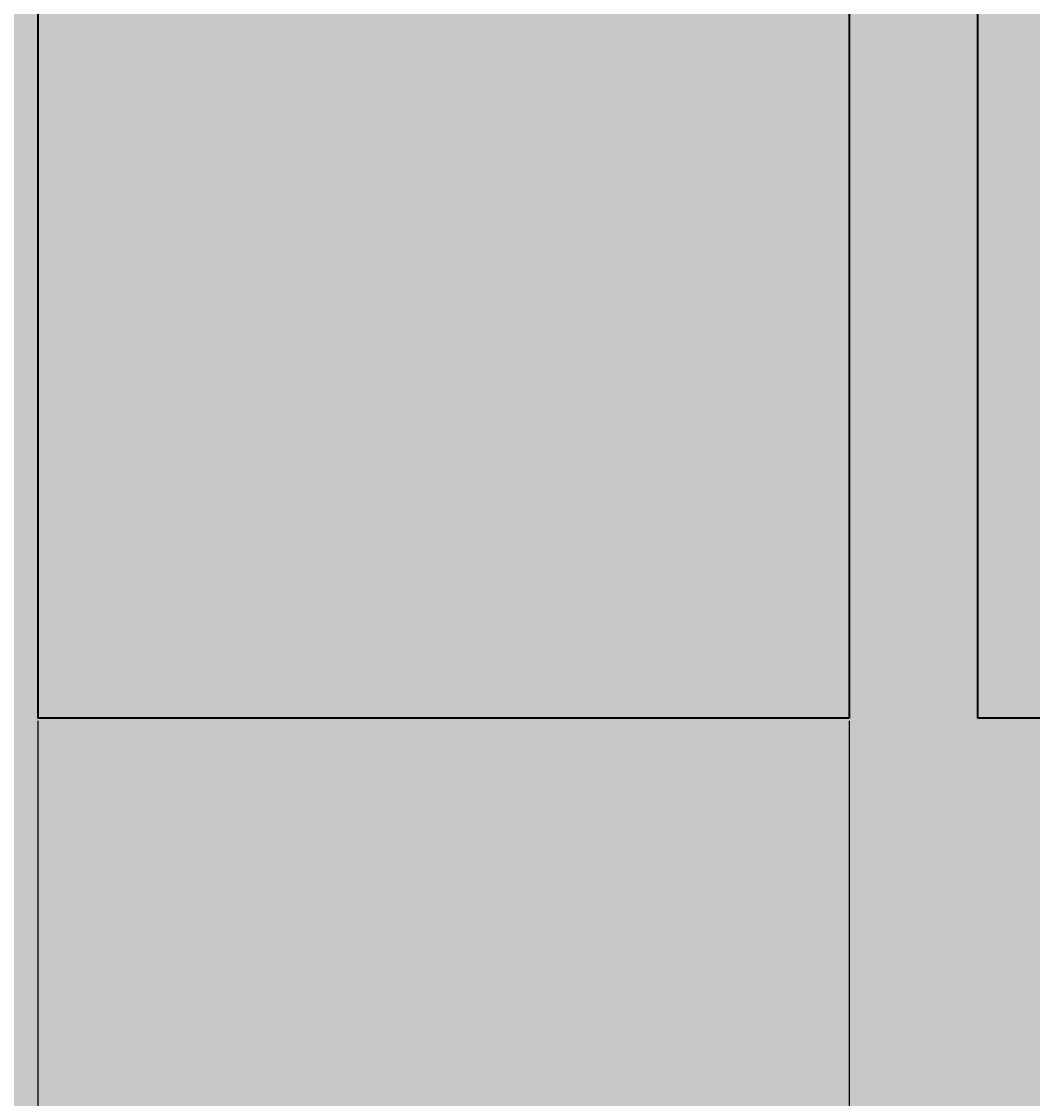
# Model space of a CAD drawing. Units: inches. Extents: x -1 to 292, y -3 to 199.
# Tile 20 of 52: x 82 to 106, y 42 to 68. Entities that reach past the tile are written whole.
import ezdxf

# ---------------------------------------------------------------- set-up
doc = ezdxf.new("R2010")
doc.units = ezdxf.units.IN
doc.header["$MEASUREMENT"] = 0
for name, color, linetype, lineweight in [('M-DIMS', 2, 'Continuous', 18), ('M-EQPM', 7, 'Continuous', 35), ('M-PATT', 8, 'Continuous', 13)]:
    doc.layers.add(name, color=color, linetype=linetype, lineweight=lineweight)
doc.styles.get("Standard").update_dxf_attribs({"font": 'arial.ttf'})
doc.dimstyles.get("Standard").update_dxf_attribs({"dimtxt": 0.18, "dimasz": 0.18, "dimexe": 0.18, "dimexo": 0.0625, "dimgap": 0.09, "dimtad": 0, "dimtih": 1, "dimtoh": 1, "dimdec": 4, "dimzin": 0, "dimdsep": 46, "dimtxsty": 'Standard', "dimcen": 0.09, "dimadec": 0, "dimazin": 0, "dimtfac": 1, "dimtdec": 4, "dimtofl": 0, "dimtmove": 0, "dimatfit": 3, "dimfxl": 1, "dimtolj": 1, "dimtzin": 0, "dimarcsym": 0})

# ---------------------------------------------------------------- blocks, each defined once
blk = doc.blocks.new('BOILER-TUBE')
blk.add_line((0, 40.63), (0, 0))
blk.add_lwpolyline([(3, 0), (0, 0)])
blk = doc.blocks.new('*D7')
at = {"layer": 'Defpoints', "color": 0, "transparency": 16777216}
for p in [(21.861, 54.582), (205.115, 54.582), (21.861, 39.982)]:
    blk.add_point(p, dxfattribs=at)
at = {"layer": 'M-DIMS', "color": 0, "lineweight": -2, "transparency": 16777216}
for p, q in [((21.861, 54.52), (21.861, 39.802)), ((205.115, 54.52), (205.115, 39.802)), ((22.041, 39.982), (113.033, 39.982)), ((204.935, 39.982), (113.944, 39.982))]:
    blk.add_line(p, q, dxfattribs=at)
at = {"layer": 'M-DIMS', "color": 0, "transparency": 16777216}
for points in [[(22.041, 40.012), (22.041, 39.952), (21.861, 39.982)], [(204.935, 40.012), (204.935, 39.952), (205.115, 39.982)]]:
    blk.add_solid(points, dxfattribs=at)
at = {"layer": 'M-DIMS', "color": 0, "transparency": 16777216, "insert": (113.488, 39.982), "char_height": 0.18, "attachment_point": 5}
blk.add_mtext('\\A1;183.25', dxfattribs=at)
blk = doc.blocks.new('*D8')
at = {"layer": 'Defpoints', "color": 0, "transparency": 16777216}
for p in [(-0.662, 126.765), (111.488, 126.765), (69.013, 25.514)]:
    blk.add_point(p, dxfattribs=at)
at = {"layer": 'M-DIMS', "color": 0, "lineweight": -2, "transparency": 16777216}
for p, q in [((111.426, 126.765), (-0.842, 126.765)), ((-0.662, 126.585), (-0.662, 76.321)), ((-0.662, 25.694), (-0.662, 75.958)), ((68.951, 25.514), (-0.842, 25.514))]:
    blk.add_line(p, q, dxfattribs=at)
at = {"layer": 'M-DIMS', "color": 0, "transparency": 16777216}
for points in [[(-0.692, 126.585), (-0.632, 126.585), (-0.662, 126.765)], [(-0.692, 25.694), (-0.632, 25.694), (-0.662, 25.514)]]:
    blk.add_solid(points, dxfattribs=at)
at = {"layer": 'M-DIMS', "color": 0, "transparency": 16777216, "insert": (-0.662, 76.14), "char_height": 0.18, "attachment_point": 5}
blk.add_mtext('\\A1;101.25', dxfattribs=at)
blk = doc.blocks.new('*D21')
at = {"layer": 'Defpoints', "color": 0, "transparency": 16777216}
for p in [(82.679, 51.267), (101.679, 51.267), (101.679, -2.71)]:
    blk.add_point(p, dxfattribs=at)
at = {"layer": 'M-DIMS', "color": 0, "lineweight": -2, "transparency": 16777216}
for p, q in [((82.679, 51.205), (82.679, -2.89)), ((101.679, 51.205), (101.679, -2.89)), ((82.859, -2.71), (91.968, -2.71)), ((101.499, -2.71), (92.389, -2.71))]:
    blk.add_line(p, q, dxfattribs=at)
at = {"layer": 'M-DIMS', "color": 0, "transparency": 16777216}
for points in [[(82.859, -2.68), (82.859, -2.74), (82.679, -2.71)], [(101.499, -2.68), (101.499, -2.74), (101.679, -2.71)]]:
    blk.add_solid(points, dxfattribs=at)
at = {"layer": 'M-DIMS', "color": 0, "transparency": 16777216, "insert": (92.179, -2.71), "char_height": 0.18, "attachment_point": 5}
blk.add_mtext('\\A1;19', dxfattribs=at)
blk = doc.blocks.new('*D22')
at = {"layer": 'Defpoints', "color": 0, "transparency": 16777216}
for p in [(82.679, 51.267), (122.679, 51.267), (122.679, -2.71)]:
    blk.add_point(p, dxfattribs=at)
at = {"layer": 'M-DIMS', "color": 0, "lineweight": -2, "transparency": 16777216}
for p, q in [((82.679, 51.205), (82.679, -2.89)), ((122.679, 51.205), (122.679, -2.89)), ((82.859, -2.71), (102.457, -2.71)), ((122.499, -2.71), (102.901, -2.71))]:
    blk.add_line(p, q, dxfattribs=at)
at = {"layer": 'M-DIMS', "color": 0, "transparency": 16777216}
for points in [[(82.859, -2.68), (82.859, -2.74), (82.679, -2.71)], [(122.499, -2.68), (122.499, -2.74), (122.679, -2.71)]]:
    blk.add_solid(points, dxfattribs=at)
at = {"layer": 'M-DIMS', "color": 0, "transparency": 16777216, "insert": (102.679, -2.71), "char_height": 0.18, "attachment_point": 5}
blk.add_mtext('\\A1;40', dxfattribs=at)

msp = doc.modelspace()

# ---------------------------------------------------------------- hatches: boundary and pattern name
at = {"layer": 'M-PATT'}
h = msp.add_hatch(color=256, dxfattribs=at)
h.set_gradient(color1=(237, 31, 36), color2=(242, 113, 114), tint=1, name='CYLINDER')
h.paths.add_polyline_path([(106.0735, 105.9941), (106.0735, 106.9941), (108.0603, 106.9941), (107.8488, 107.6501), (57.8007, 107.6501, 0.4142136), (49.9241, 99.7735), (52.3176, 101.3278), (55.0097, 99.7735), (57.4032, 101.3278), (60.0953, 99.7735), (62.4888, 101.3278), (65.1809, 99.7735), (67.5744, 101.3278), (70.2665, 99.7735), (72.66, 101.3278), (75.3521, 99.7735), (77.7456, 101.3278), (80.4377, 99.7735), (82.8312, 101.3278), (85.5233, 99.7735), (87.9168, 101.3278), (90.6089, 99.7735), (93.0024, 101.3278), (95.6945, 99.7735), (98.088, 101.3278), (100.7801, 99.7735), (103.1736, 101.3278), (105.8657, 99.7735), (108.2592, 101.3278), (110.9513, 99.7735), (113.3448, 101.3278), (116.0369, 99.7735), (118.4304, 101.3278), (121.1225, 99.7735), (123.516, 101.3278), (126.2082, 99.7735), (128.6016, 101.3278), (131.2938, 99.7735), (133.6872, 101.3278), (136.3794, 99.7735), (138.7728, 101.3278), (141.465, 99.7735), (143.8584, 101.3278), (146.5506, 99.7735), (148.944, 101.3278), (151.6362, 99.7735), (154.0296, 101.3278), (156.7218, 99.7735), (159.1152, 101.3278), (160.6222, 100.4578), (160.6222, 107.6501), (115.4883, 107.6501), (115.4883, 106.9941), (120.9032, 106.9941), (120.9032, 105.9941), (120.9032, 103.3981), (106.0735, 103.3981)])
h.paths.add_polyline_path([(169.176, 107.6501), (162.1623, 107.6501), (162.1623, 100.004), (164.2008, 101.3278), (166.893, 99.7735), (169.2864, 101.3278), (171.9786, 99.7735), (174.372, 101.3278), (177.0526, 99.7802, 0.4139642)])
h.paths.add_polyline_path([(111.4883, 107.6501), (107.8488, 107.6501), (108.0603, 106.9941), (111.4883, 106.9941)], flags=17)
h.paths.add_polyline_path([(61.6788, 91.897), (57.8007, 91.897, -0.1099266), (54.4604, 92.6403), (43.2011, 92.6403), (23.9502, 84.4688), (23.9502, 58.376), (43.2011, 47.2615), (50.9409, 47.2615, -0.2705926), (57.8007, 51.2672), (61.6788, 51.2672)])
h.paths.add_polyline_path([(73.6788, 91.897), (70.6788, 91.897), (70.6788, 51.2672), (73.6788, 51.2672)])
h.paths.add_polyline_path([(79.6788, 91.897), (76.6788, 91.897), (76.6788, 51.2672), (79.6788, 51.2672)])
h.paths.add_polyline_path([(67.6788, 91.897), (64.6788, 91.897), (64.6788, 51.2672), (67.6788, 51.2672)])
h.paths.add_polyline_path([(101.6788, 91.897), (82.6788, 91.897), (82.6788, 51.2672), (101.6788, 51.2672)])
h.paths.add_polyline_path([(107.6788, 91.897), (104.6788, 91.897), (104.6788, 51.2672), (107.6788, 51.2672)])
h.paths.add_polyline_path([(113.6788, 91.897), (110.6788, 91.897), (110.6788, 51.2672), (113.6788, 51.2672)])
h.paths.add_polyline_path([(119.6788, 91.897), (116.6788, 91.897), (116.6788, 51.2672), (119.6788, 51.2672)])
h.paths.add_polyline_path([(141.6788, 91.897), (122.6788, 91.897), (122.6788, 51.2672), (141.6788, 51.2672)])
h.paths.add_polyline_path([(147.6788, 91.897), (144.6788, 91.897), (144.6788, 51.2672), (147.6788, 51.2672)])
h.paths.add_polyline_path([(153.6788, 91.897), (150.6788, 91.897), (150.6788, 51.2672), (153.6788, 51.2672)])
h.paths.add_polyline_path([(159.6788, 91.897), (156.6788, 91.897), (156.6788, 51.2672), (159.6788, 51.2672)])
h.paths.add_polyline_path([(179.5897, 92.6403), (172.5163, 92.6403, -0.1099266), (169.176, 91.897), (162.6788, 91.897), (162.6788, 51.2672), (169.176, 51.2672, -0.2705926), (176.0358, 47.2615), (179.5897, 47.2615)])
h.paths.add_polyline_path([(203.0265, 84.4688), (183.7755, 92.6403), (181.5897, 92.6403), (181.5897, 47.2615), (183.7755, 47.2615), (203.0265, 58.376)])
h.paths.add_polyline_path([(184.4188, 61.52), (200.7224, 61.52), (200.7224, 77.7532), (184.4188, 77.7532)], flags=24)
h = msp.add_hatch(color=256, dxfattribs=at)
h.set_gradient(color1=(0, 255, 255), color2=(0, 255, 255), tint=1)
h.paths.add_polyline_path([(75.3521, 99.7735), (72.66, 101.3278), (70.2665, 99.7735), (67.5744, 101.3278), (65.1809, 99.7735), (62.4888, 101.3278), (60.0953, 99.7735), (57.4032, 101.3278), (55.0097, 99.7735), (52.3176, 101.3278), (49.9241, 99.7735, 0.4142136), (57.8007, 91.897), (61.6788, 91.897), (61.6788, 51.2672), (57.8007, 51.2672, 0.8088808), (54.5813, 36.2021), (65.0947, 51.2672), (64.6788, 51.2672), (64.6788, 91.897), (67.6788, 91.897), (67.6788, 51.2672), (65.0947, 51.2672), (54.5813, 36.2021, 0.1056561), (57.8007, 35.5141), (169.176, 35.5141, 1), (169.176, 51.2672), (162.6788, 51.2672), (162.6788, 91.897), (169.176, 91.897, 0.4144629), (177.0526, 99.7802), (174.372, 101.3278), (171.9786, 99.7735), (169.2864, 101.3278), (166.893, 99.7735), (164.2008, 101.3278), (162.1623, 100.004), (162.1623, 96.1027), (160.6222, 96.1027), (160.6222, 100.4578), (159.1152, 101.3278), (156.7218, 99.7735), (154.0296, 101.3278), (151.6362, 99.7735), (148.944, 101.3278), (146.5506, 99.7735), (143.8584, 101.3278), (141.465, 99.7735), (138.7728, 101.3278), (136.3794, 99.7735), (133.6872, 101.3278), (131.2938, 99.7735), (128.6016, 101.3278), (126.2082, 99.7735), (123.516, 101.3278), (121.1225, 99.7735), (118.4304, 101.3278), (116.0369, 99.7735), (113.3448, 101.3278), (110.9513, 99.7735), (108.2592, 101.3278), (105.8657, 99.7735), (103.1736, 101.3278), (100.7801, 99.7735), (98.088, 101.3278), (95.6945, 99.7735), (93.0024, 101.3278), (90.6089, 99.7735), (87.9168, 101.3278), (85.5233, 99.7735), (82.8312, 101.3278), (80.4377, 99.7735), (77.7456, 101.3278)])
h.paths.add_polyline_path([(79.6788, 91.897), (79.6788, 51.2672), (76.6788, 51.2672), (76.6788, 91.897)], flags=16)
h.paths.add_polyline_path([(73.6788, 91.897), (73.6788, 51.2672), (70.6788, 51.2672), (70.6788, 91.897)], flags=16)
h.paths.add_polyline_path([(82.6788, 91.897), (101.6788, 91.897), (101.6788, 51.2672), (82.6788, 51.2672)], flags=16)
h.paths.add_polyline_path([(104.6788, 91.897), (107.6788, 91.897), (107.6788, 51.2672), (104.6788, 51.2672)], flags=16)
h.paths.add_polyline_path([(110.6788, 91.897), (113.6788, 91.897), (113.6788, 51.2672), (110.6788, 51.2672)], flags=16)
h.paths.add_polyline_path([(116.6788, 91.897), (119.6788, 91.897), (119.6788, 51.2672), (116.6788, 51.2672)], flags=16)
h.paths.add_polyline_path([(122.6788, 91.897), (141.6788, 91.897), (141.6788, 51.2672), (144.6788, 51.2672), (144.6788, 91.897), (147.6788, 91.897), (147.6788, 51.2672), (122.6788, 51.2672)], flags=16)
h.paths.add_polyline_path([(150.6788, 91.897), (153.6788, 91.897), (153.6788, 51.2672), (150.6788, 51.2672)], flags=16)
h.paths.add_polyline_path([(156.6788, 91.897), (159.6788, 91.897), (159.6788, 51.2672), (156.6788, 51.2672)], flags=16)

# ---------------------------------------------------------------- linework, layer by layer
at = {"layer": 'M-EQPM'}
for p, q in [((82.6788, 91.897), (82.6788, 51.2672)), ((101.6788, 91.897), (101.6788, 51.2672))]:
    msp.add_line(p, q, dxfattribs=at)
msp.add_lwpolyline([(101.6788, 51.2672), (82.6788, 51.2672)], dxfattribs=at)

# ---------------------------------------------------------------- block references
msp.add_blockref('BOILER-TUBE', (104.679, 51.267), dxfattribs=at)

# ---------------------------------------------------------------- dimensions: what is measured, and where the dimension line sits
at = {"layer": 'M-DIMS'}
for base, p1, p2, angle, picture, middle in [((-0.6625, 126.765), (69.013, 25.5141), (111.4883, 126.765), 90, '*D8', (-0.6625, 76.1396)), ((21.8612, 39.9821), (205.1155, 54.5821), (21.8612, 54.5821), 180, '*D7', (113.4883, 39.9821))]:
    dim = msp.add_linear_dim(base=base, p1=p1, p2=p2, angle=angle, dimstyle='Standard', override={"dimdec": 2, "dimlfac": 1, "dimrnd": 0, "dimzin": 0, "dimdsep": 46, "dimlunit": 2}, dxfattribs=at)
    dim.commit()
    dim.dimension.update_dxf_attribs({"geometry": picture, "text_midpoint": middle})
for base, p2, picture, middle in [((101.6788, -2.7104), (101.6788, 51.2672), '*D21', (92.1788, -2.7104)), ((122.6788, -2.7104), (122.6788, 51.2672), '*D22', (102.6788, -2.7104))]:
    dim = msp.add_linear_dim(base=base, p1=(82.6788, 51.2672), p2=p2, dimstyle='Standard', override={"dimdec": 0, "dimlfac": 1, "dimrnd": 0, "dimzin": 0, "dimdsep": 46, "dimlunit": 2}, dxfattribs=at)
    dim.commit()
    dim.dimension.update_dxf_attribs({"geometry": picture, "text_midpoint": middle})

doc.saveas('drawing.dxf')
